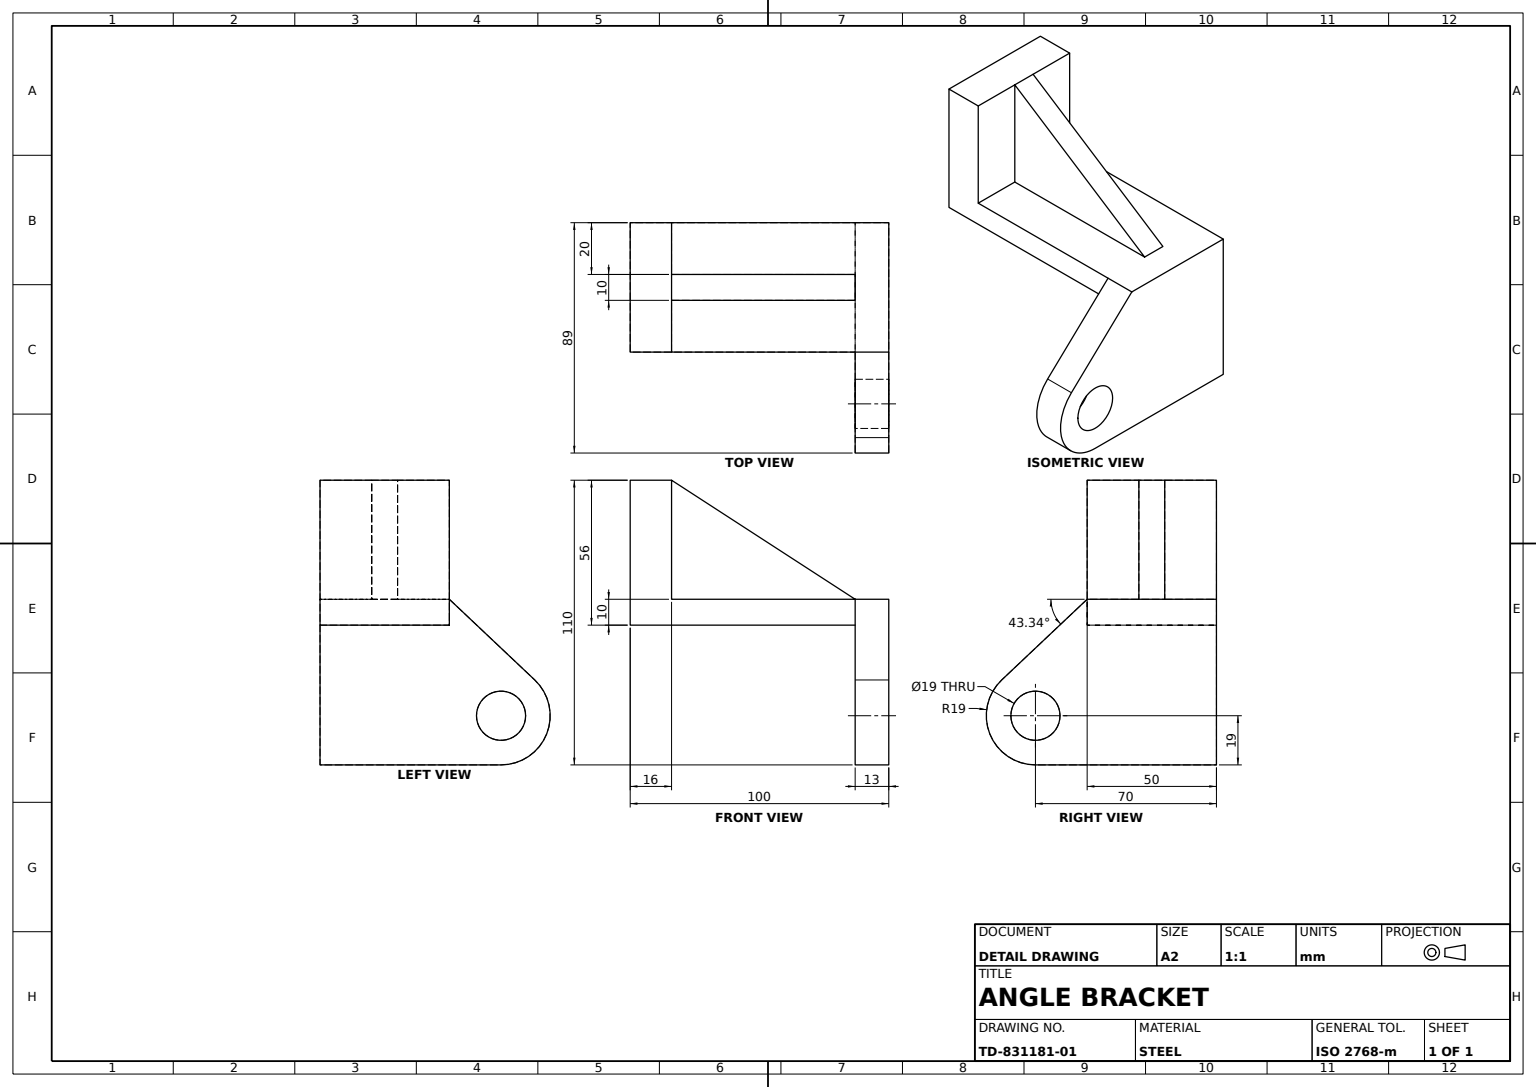
from build123d import *

# Parameters (mm, degrees)
BASE_BRACKET_DEPTH    = 50
PIVOT_LUG_DEPTH       = 13
PIVOT_HOLE_SKETCH_R   = 9.5
PIVOT_HOLE_19_DEPTH   = 13
GUSSET_DEPTH          = 30
GUSSET_TRIM_CUT_DEPTH = 20


with BuildPart() as part:
    # Base Profile Sketch → Base Bracket (new body)
    with BuildSketch(Plane.XY):
        Polygon((0, 0), (16, 0), (100, 0), (100, 10), (16, 10), (16, 56), (0, 56), align=None)
    extrude(amount=BASE_BRACKET_DEPTH)

    # Pivot Lug Sketch → Pivot Lug (add)
    with BuildSketch(Plane(origin=(100, 0, 0), x_dir=(0, 0, -1), z_dir=(1, 0, 0))):
        with BuildLine():
            Line((0, -54), (0, 10))
            Line((0, 10), (-50, 10))
            Line((-50, 10), (-83.040714674, -21.181904589))
            ThreePointArc((-83.040714674, -21.181904589), (-87.657063924, -42.016273484), (-70, -54))
            Line((-70, -54), (0, -54))
        make_face()
    extrude(amount=-PIVOT_LUG_DEPTH)

    # Pivot Hole Sketch → Pivot Hole Ø19 (cut)
    with BuildSketch(Plane(origin=(100, 0, 0), x_dir=(0, 0, -1), z_dir=(1, 0, 0))):
        with Locations((-70, -35)):
            Circle(PIVOT_HOLE_SKETCH_R)
    extrude(amount=-PIVOT_HOLE_19_DEPTH, mode=Mode.SUBTRACT)

    # Gusset Sketch → Gusset (add)
    with BuildSketch(Plane.XY.offset(50)):
        Polygon((16, 56), (16, 10), (87, 10), align=None)
    extrude(amount=-GUSSET_DEPTH)

    # Gusset Trim Sketch → Gusset Trim Cut (cut)
    with BuildSketch(Plane.XY.offset(50)):
        Polygon((16, 56), (16, 10), (87, 10), align=None)
    extrude(amount=-GUSSET_TRIM_CUT_DEPTH, mode=Mode.SUBTRACT)


solid = part.part
